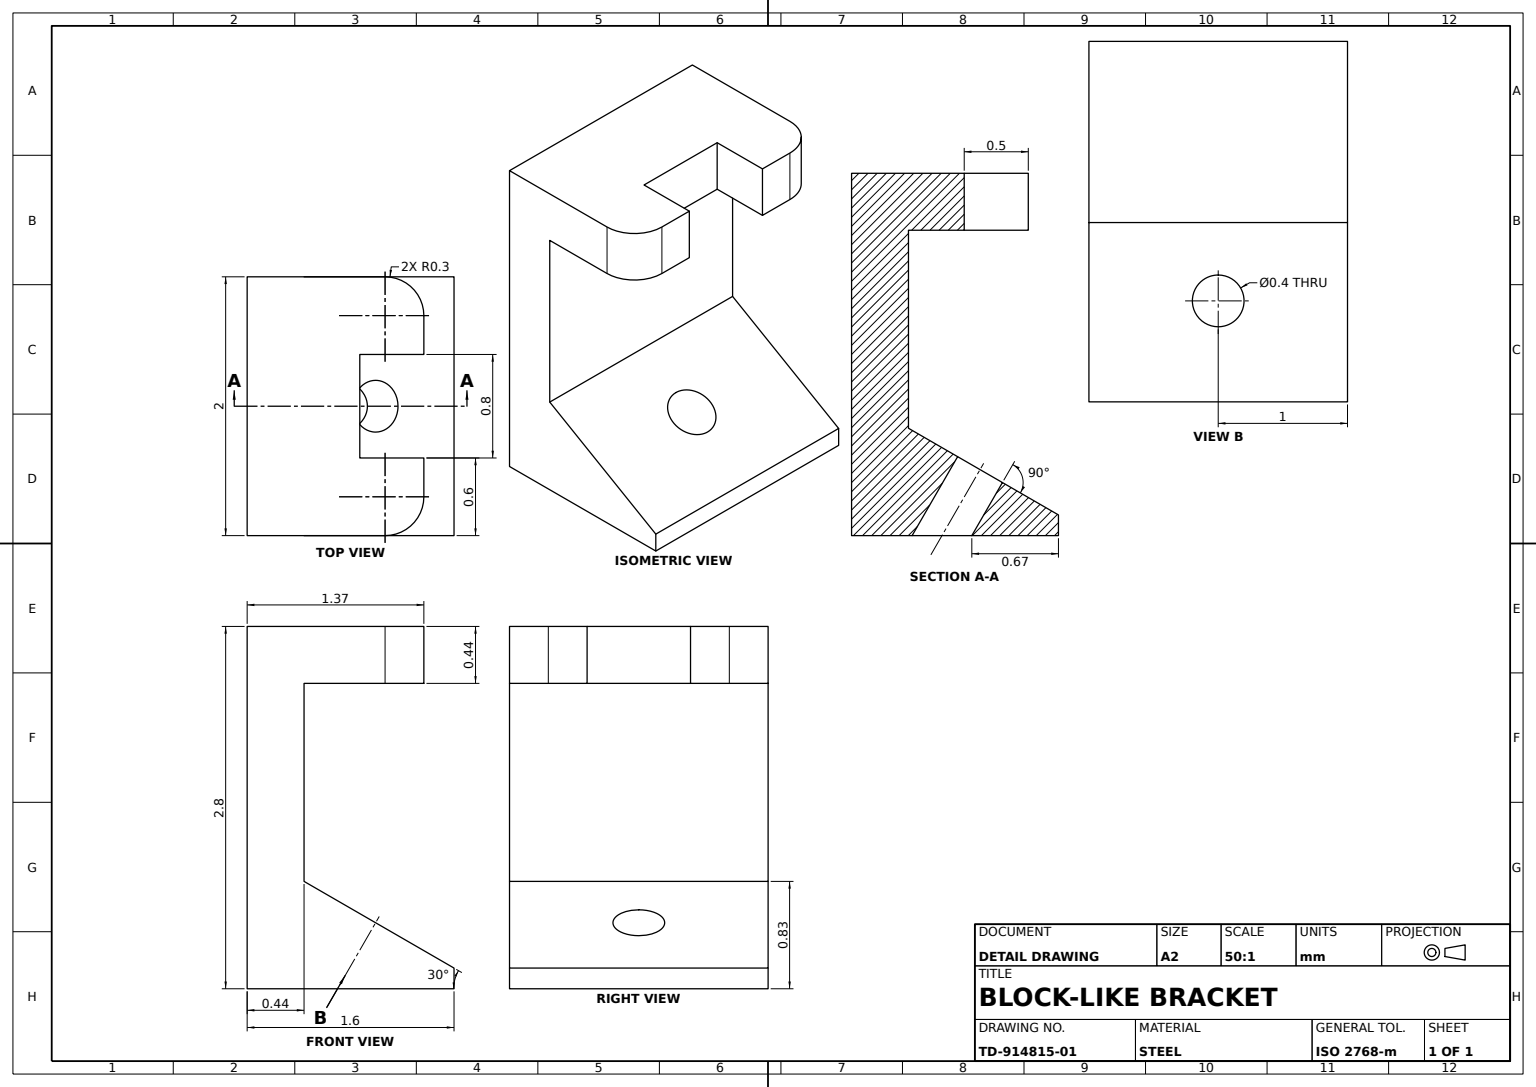
SolidWorks part; units mm, degrees
material "Plain Carbon Steel"
ref_plane "Front Plane" through (0, 0, 0) normal (0, 0, 1) x (1, 0, 0)
ref_plane "Top Plane" through (0, 0, 0) normal (0, 1, 0) x (1, 0, 0)
ref_plane "Right Plane" through (0, 0, 0) normal (1, 0, 0) x (0, 0, -1)
sketch "Bracket Profile Sketch" plane through (0, 0, 0) normal (0, 0, 1) x (1, 0, 0)
  line L0 (0, 0) -> (0, 1.4)
  line L1 (0, 1.4) -> (-1.3667, 1.4)
  line L2 (-1.3667, 1.4) -> (-1.3667, 0.96)
  line L3 (-1.3667, 0.96) -> (-0.44, 0.96)
  line L4 (-0.44, 0.96) -> (-0.44, -0.5703)
  line L5 (0, 0) -> (0, -1.4)
  line L6 (0, -1.4) -> (-1.6, -1.4)
  line L7 (-1.6, -1.4) -> (-1.6, -1.24)
  line L8 (-1.6, -1.24) -> (-0.44, -0.5703)
  line L9 (-1.6, -1.24) -> (-0.9382, -1.24) construction
  dimension "D1" = 0.44
  dimension "D2" = 1.4
  dimension "D3" = 1.4
  dimension "D4" = 1.6
  dimension "D5" = 30
  dimension "D6" = 0.44
  dimension "D7" = 1.3667
  dimension "D8" = 0.5703
extrude "Bracket Body" add sketch "Bracket Profile Sketch" along normal mid plane 2
sketch "Cut Ø0.4 Sketch" plane through (0.1369, -0.2372, 0) normal (-0.5, 0.866, 0) x (0.866, 0.5, 0)
  line L0 (-2.0056, -1) -> (-2.0056, 1) construction
  circle A0 centre (-1.3054, 0) radius 0.2
  dimension "D1" = 0.4
  dimension "D2" = 0.7003
  dimension "D3" = 1
extrude "Cut Ø0.4 Through" cut sketch "Cut Ø0.4 Sketch" against normal blind 2
sketch "Notch 0.8x0.5 Sketch" plane through (0, 1.4, 0) normal (0, 1, 0) x (1, 0, 0)
  line L0 (0, 1) -> (-0.6, 1)
  line L1 (0, 1) -> (-1.3667, 1) construction
  line L2 (-0.8712, 0.4) -> (-0.8712, -0.4)
  line L5 (-0.8712, 0.4) -> (-1.3712, 0.4)
  line L6 (-1.0689, 1) -> (-1.3667, 1)
  line L7 (-1.3667, -1) -> (-1.3667, 1) construction
  line L8 (-1.3667, -0.4) -> (-0.8712, -0.4)
  line L11 (-1.3667, 1) -> (-0.6, 1)
  line M6 (-1.3667, 1) -> (-1.3667, -1)
  dimension "D1" = 0.5
  dimension "D2" = 0.8
  dimension "D3" = 0.2978
  dimension "D4" = 0.4955
  dimension "D5" = 0.7667
  dimension "D6" = 0.6
extrude "Notch 0.8x0.5" cut sketch "Notch 0.8x0.5 Sketch" against normal blind 0.5 contours L8 L2 L5 M6
sketch "Profiled Notch Sketch" plane through (0, 1.4, 0) normal (0, 1, 0) x (1, 0, 0)
  line L0 (-1.3667, 0.7) -> (-1.3667, 1)
  line L1 (-1.3667, 1) -> (-1.0667, 1)
  line L3 (0, 0) -> (-0.5781, 0) construction
  line L4 (-1.3667, -0.7) -> (-1.3667, -1)
  line L5 (-1.3667, -1) -> (-1.0667, -1)
  arc A0 (-1.0667, 1) -> (-1.3667, 0.7) centre (-1.0667, 0.7) ccw
  arc A1 (-1.0667, -1) -> (-1.3667, -0.7) centre (-1.0667, -0.7) cw
  dimension "D1" = 0.3
  dimension "D2" = 1.2759
extrude "Profiled Notch" cut sketch "Profiled Notch Sketch" against normal blind 0.5
